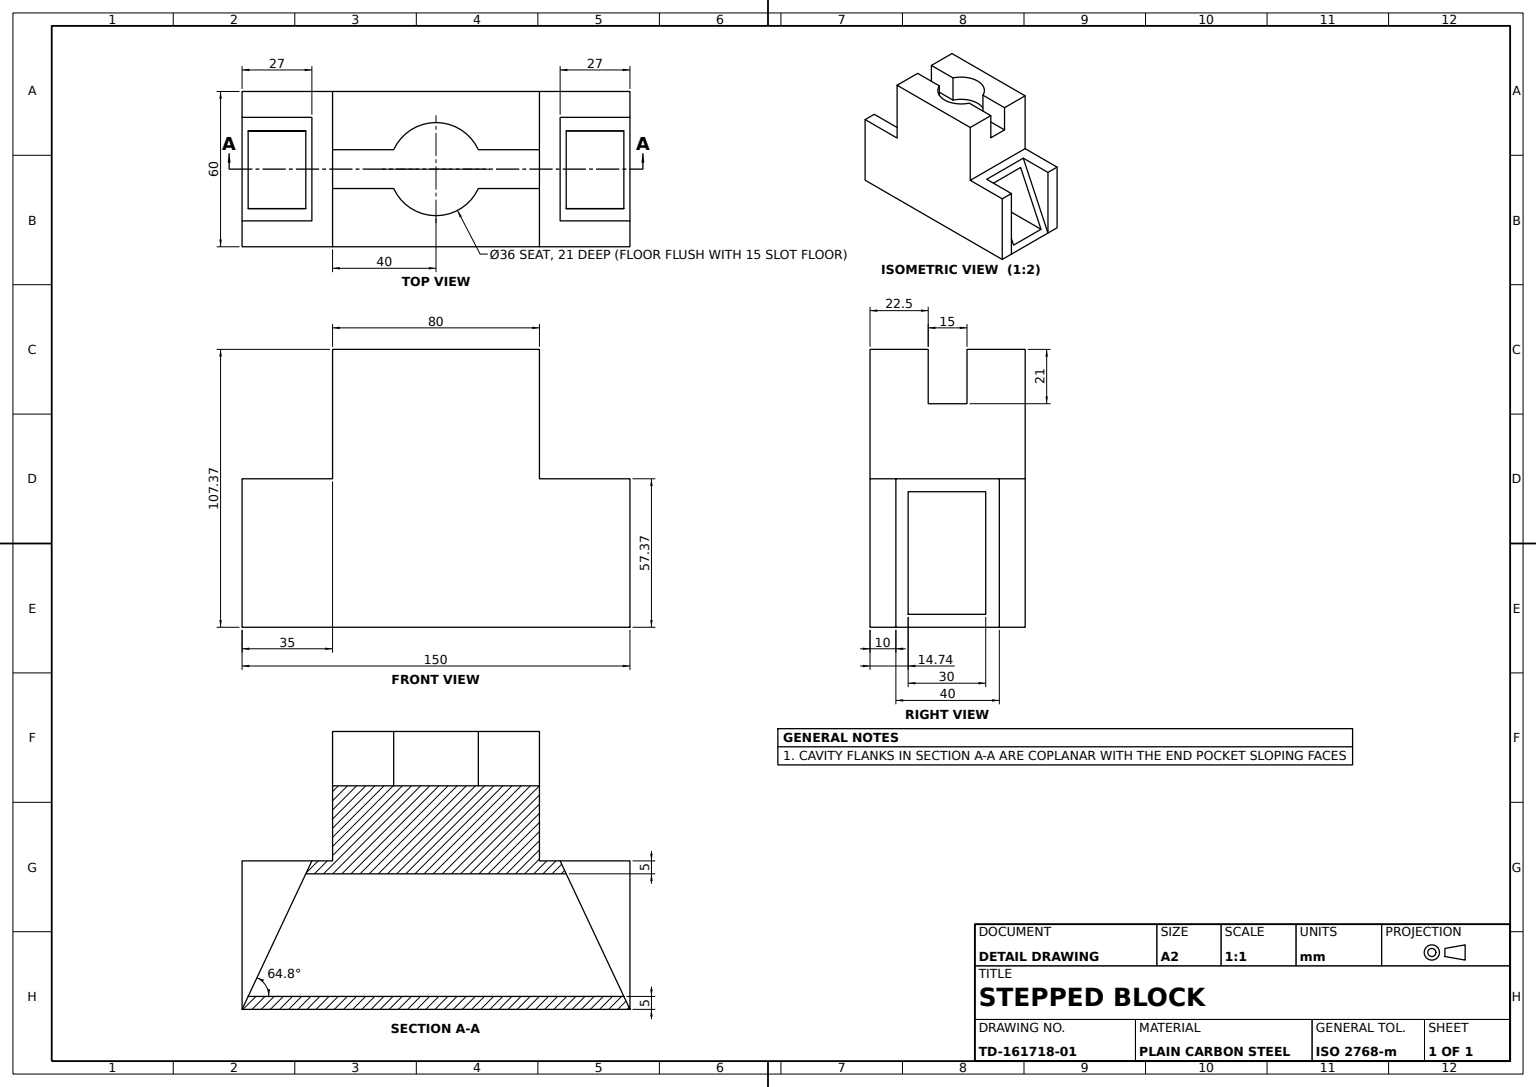
SolidWorks part; units mm, degrees
material "Plain Carbon Steel"
ref_plane "Front Plane" through (0, 0, 0) normal (0, 0, 1) x (1, 0, 0)
ref_plane "Top Plane" through (0, 0, 0) normal (0, 1, 0) x (1, 0, 0)
ref_plane "Right Plane" through (0, 0, 0) normal (1, 0, 0) x (0, 0, -1)
sketch "Base Block Profile" plane through (0, 0, 0) normal (0, 0, 1) x (1, 0, 0)
  line L0 (40, 28.6871) -> (75, 28.6871)
  line L1 (-75, 28.6871) -> (-40, 28.6871)
  line L2 (-75, 28.6871) -> (-75, -28.6871)
  line L3 (-75, -28.6871) -> (75, -28.6871)
  line L4 (75, 28.6871) -> (75, -28.6871)
  line L5 (-75, 28.6871) -> (75, -28.6871) construction
  line L6 (-75, -28.6871) -> (75, 28.6871) construction
  line L7 (-40, 78.6871) -> (40, 78.6871)
  line L8 (-40, 78.6871) -> (-40, 28.6871)
  line L10 (40, 78.6871) -> (40, 28.6871)
  point P0 (0, 0)
  dimension "D1" = 57.3741
  dimension "D2" = 150
  dimension "D3" = 50
  dimension "D4" = 80
  dimension "D5" = 35
extrude "Base Block" add sketch "Base Block Profile" against normal blind 60
sketch "Top Slot Profile" plane through (0, 78.6871, 0) normal (0, 1, 0) x (1, 0, 0)
  line L0 (-40, 60) -> (-40, 0) construction
  line L1 (-40, 37.5) -> (-16.3631, 37.5)
  line L2 (-40, 37.5) -> (-40, 22.5)
  line L3 (-40, 22.5) -> (-16.3631, 22.5)
  line L4 (40, 37.5) -> (40, 22.5)
  line L5 (40, 60) -> (40, 0) construction
  line L8 (40, 60) -> (-40, 60) construction
  line L11 (16.3631, 37.5) -> (40, 37.5)
  line L12 (16.3631, 22.5) -> (40, 22.5)
  arc A0 (-16.3631, 22.5) -> (16.3631, 22.5) centre (0, 30) ccw
  arc A1 (16.3631, 37.5) -> (-16.3631, 37.5) centre (0, 30) ccw
  dimension "D1" = 36
  dimension "D2" = 40
  dimension "D3" = 15
  dimension "D4" = 30
  dimension "D5" = 22.5
extrude "Top Slot With Bore Seat" cut sketch "Top Slot Profile" against normal blind 21
sketch "End Channel Profile" plane through (-75, 0, 0) normal (-1, 0, 0) x (0, 0, 1)
  line L0 (-60, 28.6871) -> (0, 28.6871) construction
  line L1 (-49.7406, 28.6871) -> (-9.7406, 28.6871)
  line L2 (-49.7406, 28.6871) -> (-49.7406, -28.6871)
  line L3 (-49.7406, -28.6871) -> (-9.7406, -28.6871)
  line L4 (-9.7406, 28.6871) -> (-9.7406, -28.6871)
  line L5 (-60, -28.6871) -> (0, -28.6871) construction
  line L7 (-44.7406, 23.6871) -> (-14.7406, 23.6871)
  line L8 (-44.7406, 23.6871) -> (-44.7406, -23.6871)
  line L9 (-44.7406, -23.6871) -> (-14.7406, -23.6871)
  line L10 (-14.7406, 23.6871) -> (-14.7406, -23.6871)
  dimension "D1" = 5
  dimension "D2" = 40
  dimension "D3" = 5
  dimension "D4" = 5
  dimension "D5" = 5
  dimension "D6" = 9.7406
extrude "End Channel Cut" cut sketch "End Channel Profile" against normal through all contours L8 L7 L10 L9
ref_plane "Pocket Offset Plane" through (0, 0, -10) normal (0, 0, 1) x (1, 0, 0)
sketch "Triangular Pocket Profile" plane through (0, 0, -10) normal (0, 0, 1) x (1, 0, 0)
  line L0 (-48, 28.6871) -> (-75, -28.6871)
  line L1 (-40, 28.6871) -> (-75, 28.6871) construction
  line L2 (-75, -28.6871) -> (-75, 28.6871)
  line L3 (-75, 28.6871) -> (-48, 28.6871)
  line L4 (48, 28.6871) -> (75, -28.6871)
  line L5 (75, 28.6871) -> (40, 28.6871) construction
  line L6 (75, -28.6871) -> (75, 28.6871)
  line L7 (75, 28.6871) -> (48, 28.6871)
  dimension "D1" = 27
  dimension "D2" = 27
extrude "Triangular Pocket Cut" cut sketch "Triangular Pocket Profile" against normal blind 40
